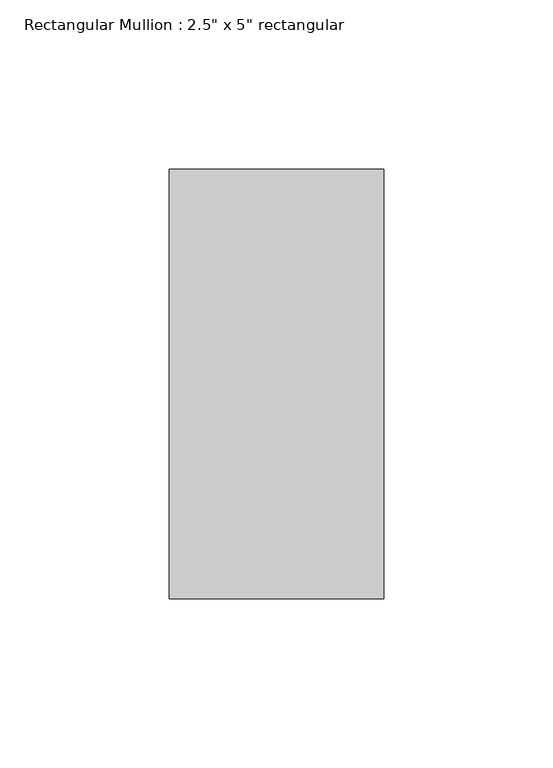
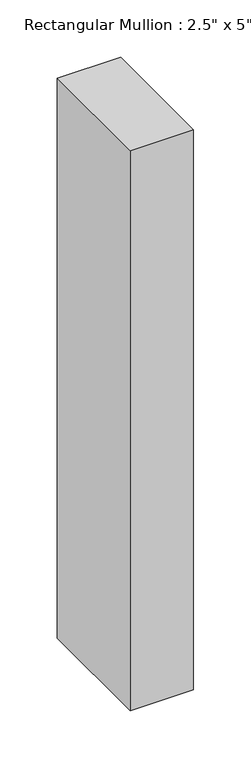
"""IFC4 building model written with IfcOpenShell, lengths in millimetres: member geometry."""

from ifc_helpers import new_model, si_unit, frame, origin, place, context, project, spatial, polyline, outline, extrude, source, transform, mapped, element, save


def member_50ab567a(model_context):
    return source(origin(), model_context, "Body", "SweptSolid", [
        extrude(outline(polyline([(31.75, 63.5), (31.75, -63.5), (-31.75, -63.5), (-31.75, 63.5), (31.75, 63.5)])), frame((0.0, 0.0, -595.5236621), z_axis=(0.0, 0.0, 1.0), x_axis=(1.0, 0.0, 0.0)), (0.0, 0.0, 1.0), 595.5236621),
    ])


if __name__ == "__main__":
    model = new_model("IFC4")
    model_context = context("Model", 3, world=origin())
    ifc_project = project(units=[si_unit("LENGTHUNIT", "METRE", prefix="MILLI")], contexts=[model_context])
    site = spatial("IfcSite", under=ifc_project)
    building = spatial("IfcBuilding", under=site)
    placement = place(None, origin())
    member_shape = member_50ab567a(model_context)
    element("IfcMember", 1, ObjectType="Rectangular Mullion : 2.5\" x 5\" rectangular", at=placement, inside=building, context=model_context, shape_type="MappedRepresentation", body=[
        mapped(member_shape, transform((0.0, 0.0, 0.0), x_axis=(1.0, 0.0, 0.0), y_axis=(0.0, 1.0, 0.0), z_axis=(0.0, 0.0, 1.0))),
    ])
    save(model, "model.ifc")

# Revit data of these elements
# Type "Rectangular Mullion : 2.5\" x 5\" rectangular"
#   built-in parameter 1007304 = 0.416667 (stored number, unit not read)
#   built-in parameter 1007301 = 0.104167 (stored number, unit not read)
#   built-in parameter 1007300 = 0.104167 (stored number, unit not read)
# Element 1 (IfcMember, "Rectangular Mullion : 2.5\" x 5\" rectangular")
#   Materials on its faces: "Aluminum"
# Materials
#   "Aluminum": class "Metal", colour RGB 247 247 247, transparency 0, Description = "Aluminum 6061", Cost = 0
